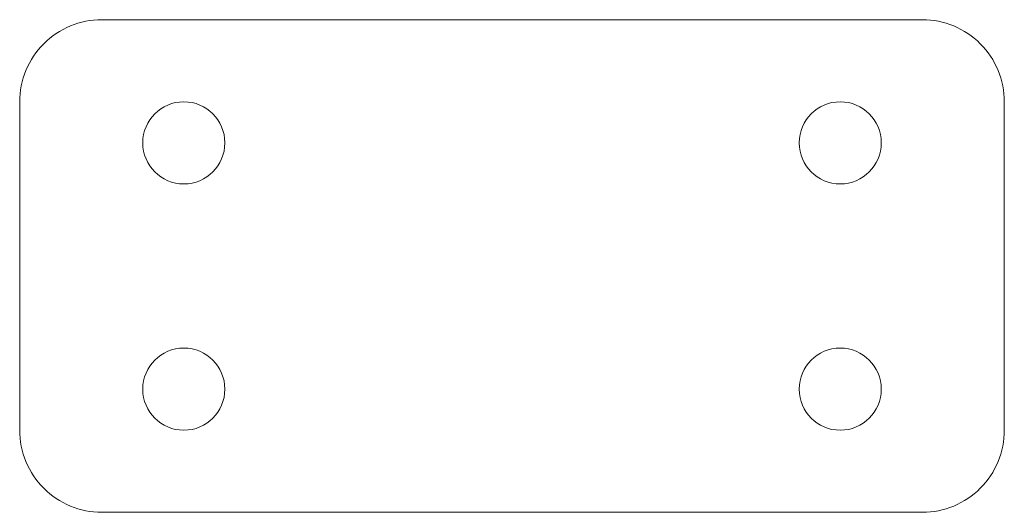
# Model space of a CAD drawing. Units: millimetres. Extents: x 2955 to 3075, y 1762 to 1822.
import ezdxf

# ---------------------------------------------------------------- set-up
doc = ezdxf.new("R2010")
doc.units = ezdxf.units.MM
doc.layers.add('M-CONS', color=8, linetype='Continuous', lineweight=18)

msp = doc.modelspace()

# ---------------------------------------------------------------- linework, layer by layer
at = {"layer": 'M-CONS'}
msp.add_lwpolyline([(3034.64, 1762.47), (3064.64, 1762.47, 0.414214), (3074.64, 1772.47), (3074.64, 1812.47, 0.414214), (3064.64, 1822.47), (2964.64, 1822.47, 0.414214), (2954.64, 1812.47), (2954.64, 1772.47, 0.414214), (2964.64, 1762.47)], format="xyb", close=True, dxfattribs=at)
for centre in [(2974.64, 1807.47), (3054.64, 1807.47), (2974.64, 1777.47), (3054.64, 1777.47)]:
    msp.add_circle(centre, 5, dxfattribs=at)

doc.saveas('drawing.dxf')
